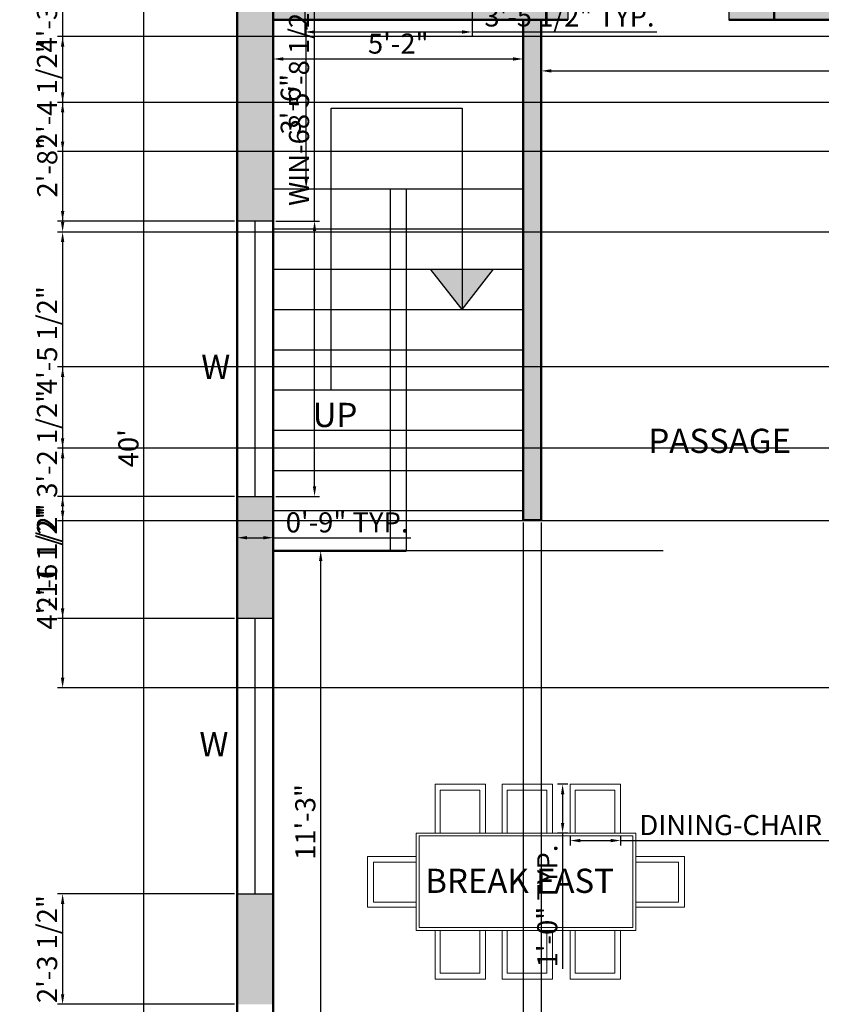
# Model space of a CAD drawing. Units: inches. Extents: x 2064 to 2999, y 1440 to 2089.
# Tile 2 of 7: x 2064 to 2263, y 1590 to 1835. Entities that reach past the tile are written whole.
import ezdxf

# ---------------------------------------------------------------- set-up
doc = ezdxf.new("R2010")
doc.units = ezdxf.units.IN
for name, color, linetype, lineweight in [('A-ANNO-DIMS', 2, 'Continuous', 18), ('A-ANNO-TEXT', 3, 'Continuous', 18), ('A-AREA-IDEN', 7, 'Continuous', 18), ('A-DOOR', 4, 'Continuous', 25), ('A-FLOR-STRS', 2, 'Continuous', 25), ('A-FURN', 8, 'Continuous', 18), ('A-GLAZ', 3, 'Continuous', 25), ('A-WALL', 7, 'Continuous', 50), ('A-WALL-PATT', 8, 'Continuous', 13)]:
    doc.layers.add(name, color=color, linetype=linetype, lineweight=lineweight)
doc.styles.get("Standard").update_dxf_attribs({"font": 'arial.ttf'})
doc.dimstyles.new('ISO-25', dxfattribs={"dimtxt": 5, "dimasz": 2.5, "dimexe": 1.25, "dimexo": 0.625, "dimtad": 1, "dimdec": 0, "dimlunit": 4, "dimtxsty": 'Standard', "dimcen": 2.5, "dimadec": 0, "dimazin": 0, "dimtfac": 1, "dimtdec": 0, "dimtmove": 0, "dimatfit": 3, "dimfxl": 1, "dimarcsym": 0})

# ---------------------------------------------------------------- blocks, each defined once
blk = doc.blocks.new('*U2')
for p, q in [((0, 0), (0, -6)), ((40, 0), (40, -6))]:
    blk.add_line(p, q)
blk.add_lwpolyline([(0, 0), (0, 40), (1.75, 40), (1.75, 0)], close=True)
blk.add_arc((0, 0), 40, 0, 90)
blk = doc.blocks.new('*D16')
at = {"layer": 'A-ANNO-DIMS', "color": 0, "lineweight": -2, "transparency": 16777216}
for p, q in [((2193.43, 1833.95), (2193.43, 1820.6)), ((2368.32, 1833.95), (2368.32, 1820.6)), ((2195.93, 1821.85), (2365.82, 1821.85))]:
    blk.add_line(p, q, dxfattribs=at)
at = {"layer": 'A-ANNO-DIMS', "color": 0, "transparency": 16777216}
for points in [[(2195.93, 1822.26), (2195.93, 1821.43), (2193.43, 1821.85)], [(2365.82, 1822.26), (2365.82, 1821.43), (2368.32, 1821.85)]]:
    blk.add_solid(points, dxfattribs=at)
at = {"layer": 'Defpoints', "color": 0, "transparency": 16777216}
for p in [(2193.43, 1834.57), (2368.32, 1834.57), (2368.32, 1821.85)]:
    blk.add_point(p, dxfattribs=at)
at = {"layer": 'A-ANNO-DIMS', "color": 0, "transparency": 16777216, "insert": (2280.88, 1824.98), "char_height": 5, "attachment_point": 5}
blk.add_mtext('14\'-7"', dxfattribs=at)
blk = doc.blocks.new('*D18')
at = {"layer": 'A-ANNO-DIMS', "color": 0, "lineweight": -2, "transparency": 16777216}
for p, q in [((2117.19, 1968.07), (2093.39, 1968.07)), ((2094.64, 1490.57), (2094.64, 1965.57)), ((2117.19, 1488.07), (2093.39, 1488.07))]:
    blk.add_line(p, q, dxfattribs=at)
at = {"layer": 'A-ANNO-DIMS', "color": 0, "transparency": 16777216}
for points in [[(2094.23, 1965.57), (2095.06, 1965.57), (2094.64, 1968.07)], [(2094.23, 1490.57), (2095.06, 1490.57), (2094.64, 1488.07)]]:
    blk.add_solid(points, dxfattribs=at)
at = {"layer": 'Defpoints', "color": 0, "transparency": 16777216}
for p in [(2094.64, 1968.07), (2117.82, 1968.07), (2117.82, 1488.07)]:
    blk.add_point(p, dxfattribs=at)
at = {"layer": 'A-ANNO-DIMS', "color": 0, "transparency": 16777216, "insert": (2091.47, 1728.07), "char_height": 5, "attachment_point": 5, "rotation": 90}
blk.add_mtext("40'", dxfattribs=at)
blk = doc.blocks.new('*D36')
at = {"layer": 'A-ANNO-DIMS', "color": 0, "lineweight": -2, "transparency": 16777216}
for p, q in [((2126.82, 1833.95), (2126.82, 1823.56)), ((2188.93, 1833.95), (2188.93, 1823.56)), ((2129.32, 1824.81), (2186.43, 1824.81))]:
    blk.add_line(p, q, dxfattribs=at)
at = {"layer": 'A-ANNO-DIMS', "color": 0, "transparency": 16777216}
for points in [[(2129.32, 1825.23), (2129.32, 1824.39), (2126.82, 1824.81)], [(2186.43, 1825.23), (2186.43, 1824.39), (2188.93, 1824.81)]]:
    blk.add_solid(points, dxfattribs=at)
at = {"layer": 'Defpoints', "color": 0, "transparency": 16777216}
for p in [(2126.82, 1834.57), (2188.93, 1834.57), (2188.93, 1824.81)]:
    blk.add_point(p, dxfattribs=at)
at = {"layer": 'A-ANNO-DIMS', "color": 0, "transparency": 16777216, "insert": (2157.88, 1827.99), "char_height": 5, "attachment_point": 5}
blk.add_mtext('5\'-2"', dxfattribs=at)
blk = doc.blocks.new('*D37')
at = {"layer": 'A-ANNO-DIMS', "color": 0, "lineweight": -2, "transparency": 16777216}
for p, q in [((2127.44, 1834.57), (2136.25, 1834.57)), ((2135, 1795.07), (2135, 1832.07)), ((2127.44, 1792.57), (2136.25, 1792.57))]:
    blk.add_line(p, q, dxfattribs=at)
at = {"layer": 'A-ANNO-DIMS', "color": 0, "transparency": 16777216}
for points in [[(2134.58, 1832.07), (2135.42, 1832.07), (2135, 1834.57)], [(2134.58, 1795.07), (2135.42, 1795.07), (2135, 1792.57)]]:
    blk.add_solid(points, dxfattribs=at)
at = {"layer": 'Defpoints', "color": 0, "transparency": 16777216}
for p in [(2126.82, 1834.57), (2135, 1834.57), (2126.82, 1792.57)]:
    blk.add_point(p, dxfattribs=at)
at = {"layer": 'A-ANNO-DIMS', "color": 0, "transparency": 16777216, "insert": (2131.82, 1813.57), "char_height": 5, "attachment_point": 5, "rotation": 90}
blk.add_mtext('3\'-6"', dxfattribs=at)
blk = doc.blocks.new('*D39')
at = {"layer": 'A-ANNO-DIMS', "color": 0, "lineweight": -2, "transparency": 16777216}
for p, q in [((2223.69, 1702.57), (2137.36, 1702.57)), ((2138.61, 1570.34), (2138.61, 1700.07)), ((2223.69, 1567.84), (2137.36, 1567.84))]:
    blk.add_line(p, q, dxfattribs=at)
at = {"layer": 'A-ANNO-DIMS', "color": 0, "transparency": 16777216}
for points in [[(2138.19, 1700.07), (2139.03, 1700.07), (2138.61, 1702.57)], [(2138.19, 1570.34), (2139.03, 1570.34), (2138.61, 1567.84)]]:
    blk.add_solid(points, dxfattribs=at)
at = {"layer": 'Defpoints', "color": 0, "transparency": 16777216}
for p in [(2138.61, 1702.57), (2224.32, 1702.57), (2224.32, 1567.84)]:
    blk.add_point(p, dxfattribs=at)
at = {"layer": 'A-ANNO-DIMS', "color": 0, "transparency": 16777216, "insert": (2135.43, 1635.2), "char_height": 5, "attachment_point": 5, "rotation": 90}
blk.add_mtext('11\'-3"', dxfattribs=at)
blk = doc.blocks.new('DINING-CHAIR')
for p, q in [((0, 0), (0, 12.53)), ((0, 12.53), (12.13, 12.53)), ((12.13, 0), (0, 0))]:
    blk.add_line(p, q)
blk.add_lwpolyline([(12.13, 11.12), (1.51, 11.12), (1.51, 1.24), (12.13, 1.24)], close=True)
blk = doc.blocks.new('WIN-68')
blk.add_line((4.5, 0), (4.5, 68.43))
blk.add_lwpolyline([(0, 0), (9, 0), (9, 68.43), (0, 68.43)], close=True)
blk = doc.blocks.new('*D50')
at = {"layer": 'A-ANNO-DIMS', "color": 0, "lineweight": -2, "transparency": 16777216}
for p, q in [((2134.69, 1838.45), (2134.69, 1830.27)), ((2176.26, 1838.45), (2176.26, 1830.27)), ((2137.19, 1831.52), (2173.76, 1831.52)), ((2176.26, 1831.52), (2222.13, 1831.52))]:
    blk.add_line(p, q, dxfattribs=at)
at = {"layer": 'A-ANNO-DIMS', "color": 0, "transparency": 16777216}
for points in [[(2137.19, 1831.93), (2137.19, 1831.1), (2134.69, 1831.52)], [(2173.76, 1831.93), (2173.76, 1831.1), (2176.26, 1831.52)]]:
    blk.add_solid(points, dxfattribs=at)
at = {"layer": 'Defpoints', "color": 0, "transparency": 16777216}
for p in [(2134.69, 1839.07), (2176.26, 1839.07), (2176.26, 1831.52)]:
    blk.add_point(p, dxfattribs=at)
at = {"layer": 'A-ANNO-DIMS', "color": 0, "transparency": 16777216, "insert": (2200.44, 1834.73), "char_height": 5, "attachment_point": 5}
blk.add_mtext('3\'-5 1/2" TYP.', dxfattribs=at)
blk = doc.blocks.new('*D57')
at = {"layer": 'A-ANNO-DIMS', "color": 0, "lineweight": -2, "transparency": 16777216}
for p, q in [((2200.61, 1631.83), (2200.61, 1629.33)), ((2203.11, 1630.58), (2210.65, 1630.58)), ((2213.15, 1631.83), (2213.15, 1629.33)), ((2213.15, 1630.58), (2309.22, 1630.58))]:
    blk.add_line(p, q, dxfattribs=at)
at = {"layer": 'A-ANNO-DIMS', "color": 0, "transparency": 16777216}
for points in [[(2203.11, 1631), (2203.11, 1630.16), (2200.61, 1630.58)], [(2210.65, 1631), (2210.65, 1630.16), (2213.15, 1630.58)]]:
    blk.add_solid(points, dxfattribs=at)
at = {"layer": 'Defpoints', "color": 0, "transparency": 16777216}
for p in [(2200.61, 1632.46), (2213.15, 1632.46), (2213.15, 1630.58)]:
    blk.add_point(p, dxfattribs=at)
at = {"layer": 'A-ANNO-DIMS', "color": 0, "transparency": 16777216, "insert": (2262.43, 1633.79), "char_height": 5, "attachment_point": 5}
blk.add_mtext('DINING-CHAIR 1\'-0 1/2" TYP.', dxfattribs=at)
blk = doc.blocks.new('*D58')
at = {"layer": 'A-ANNO-DIMS', "color": 0, "lineweight": -2, "transparency": 16777216}
for p, q in [((2199.99, 1644.59), (2197.48, 1644.59)), ((2198.73, 1642.09), (2198.73, 1634.96)), ((2199.99, 1632.46), (2197.48, 1632.46)), ((2198.73, 1632.46), (2198.73, 1598.7))]:
    blk.add_line(p, q, dxfattribs=at)
at = {"layer": 'A-ANNO-DIMS', "color": 0, "transparency": 16777216}
for points in [[(2198.32, 1642.09), (2199.15, 1642.09), (2198.73, 1644.59)], [(2198.32, 1634.96), (2199.15, 1634.96), (2198.73, 1632.46)]]:
    blk.add_solid(points, dxfattribs=at)
at = {"layer": 'Defpoints', "color": 0, "transparency": 16777216}
for p in [(2200.61, 1644.59), (2198.73, 1632.46), (2200.61, 1632.46)]:
    blk.add_point(p, dxfattribs=at)
at = {"layer": 'A-ANNO-DIMS', "color": 0, "transparency": 16777216, "insert": (2195.56, 1614.33), "char_height": 5, "attachment_point": 5, "rotation": 90}
blk.add_mtext('1\'-0" TYP.', dxfattribs=at)
blk = doc.blocks.new('*D59')
at = {"layer": 'A-ANNO-DIMS', "color": 0, "lineweight": -2, "transparency": 16777216}
for p, q in [((2137.08, 1784.53), (2137.08, 1856.23)), ((2127.44, 1784.53), (2138.33, 1784.53)), ((2137.08, 1718.6), (2137.08, 1782.03)), ((2127.44, 1716.1), (2138.33, 1716.1))]:
    blk.add_line(p, q, dxfattribs=at)
at = {"layer": 'A-ANNO-DIMS', "color": 0, "transparency": 16777216}
for points in [[(2136.67, 1782.03), (2137.5, 1782.03), (2137.08, 1784.53)], [(2136.67, 1718.6), (2137.5, 1718.6), (2137.08, 1716.1)]]:
    blk.add_solid(points, dxfattribs=at)
at = {"layer": 'Defpoints', "color": 0, "transparency": 16777216}
for p in [(2126.82, 1784.53), (2137.08, 1784.53), (2126.82, 1716.1)]:
    blk.add_point(p, dxfattribs=at)
at = {"layer": 'A-ANNO-DIMS', "color": 0, "transparency": 16777216, "insert": (2133.87, 1821.63), "char_height": 5, "attachment_point": 5, "rotation": 90}
blk.add_mtext('WIN-68 5\'-8 1/2" TYP.', dxfattribs=at)
blk = doc.blocks.new('*D60')
at = {"layer": 'A-ANNO-DIMS', "color": 0, "lineweight": -2, "transparency": 16777216}
for p, q in [((2117.82, 1715.48), (2117.82, 1704.59)), ((2126.82, 1715.48), (2126.82, 1704.59)), ((2120.32, 1705.84), (2124.32, 1705.84)), ((2126.82, 1705.84), (2161.05, 1705.84))]:
    blk.add_line(p, q, dxfattribs=at)
at = {"layer": 'A-ANNO-DIMS', "color": 0, "transparency": 16777216}
for points in [[(2120.32, 1706.25), (2120.32, 1705.42), (2117.82, 1705.84)], [(2124.32, 1706.25), (2124.32, 1705.42), (2126.82, 1705.84)]]:
    blk.add_solid(points, dxfattribs=at)
at = {"layer": 'Defpoints', "color": 0, "transparency": 16777216}
for p in [(2117.82, 1716.1), (2126.82, 1716.1), (2126.82, 1705.84)]:
    blk.add_point(p, dxfattribs=at)
at = {"layer": 'A-ANNO-DIMS', "color": 0, "transparency": 16777216, "insert": (2145.18, 1709.01), "char_height": 5, "attachment_point": 5}
blk.add_mtext('0\'-9" TYP.', dxfattribs=at)
blk = doc.blocks.new('*D70')
at = {"layer": 'A-ANNO-DIMS', "color": 0, "lineweight": -2, "transparency": 16777216}
for p, q in [((2477.19, 1865.66), (2073.22, 1865.66)), ((2074.47, 1863.16), (2074.47, 1816.51)), ((2477.19, 1814.01), (2073.22, 1814.01))]:
    blk.add_line(p, q, dxfattribs=at)
at = {"layer": 'A-ANNO-DIMS', "color": 0, "transparency": 16777216}
for points in [[(2074.05, 1863.16), (2074.89, 1863.16), (2074.47, 1865.66)], [(2074.05, 1816.51), (2074.89, 1816.51), (2074.47, 1814.01)]]:
    blk.add_solid(points, dxfattribs=at)
at = {"layer": 'Defpoints', "color": 0, "transparency": 16777216}
for p in [(2477.82, 1865.66), (2074.47, 1814.01), (2477.82, 1814.01)]:
    blk.add_point(p, dxfattribs=at)
at = {"layer": 'A-ANNO-DIMS', "color": 0, "transparency": 16777216, "insert": (2071.26, 1839.83), "char_height": 5, "attachment_point": 5, "rotation": 90}
blk.add_mtext('4\'-3 1/2"', dxfattribs=at)
blk = doc.blocks.new('*D71')
at = {"layer": 'A-ANNO-DIMS', "color": 0, "lineweight": -2, "transparency": 16777216}
for p, q in [((2477.19, 1814.01), (2073.22, 1814.01)), ((2074.47, 1811.51), (2074.47, 1784.3)), ((2477.19, 1781.8), (2073.22, 1781.8))]:
    blk.add_line(p, q, dxfattribs=at)
at = {"layer": 'A-ANNO-DIMS', "color": 0, "transparency": 16777216}
for points in [[(2074.05, 1811.51), (2074.89, 1811.51), (2074.47, 1814.01)], [(2074.05, 1784.3), (2074.89, 1784.3), (2074.47, 1781.8)]]:
    blk.add_solid(points, dxfattribs=at)
at = {"layer": 'Defpoints', "color": 0, "transparency": 16777216}
for p in [(2477.82, 1814.01), (2074.47, 1781.8), (2477.82, 1781.8)]:
    blk.add_point(p, dxfattribs=at)
at = {"layer": 'A-ANNO-DIMS', "color": 0, "transparency": 16777216, "insert": (2071.29, 1797.91), "char_height": 5, "attachment_point": 5, "rotation": 90}
blk.add_mtext('2\'-8"', dxfattribs=at)
blk = doc.blocks.new('*D72')
at = {"layer": 'A-ANNO-DIMS', "color": 0, "lineweight": -2, "transparency": 16777216}
for p, q in [((2477.19, 1781.8), (2073.22, 1781.8)), ((2074.47, 1779.3), (2074.47, 1730.57)), ((2477.19, 1728.07), (2073.22, 1728.07))]:
    blk.add_line(p, q, dxfattribs=at)
at = {"layer": 'A-ANNO-DIMS', "color": 0, "transparency": 16777216}
for points in [[(2074.05, 1779.3), (2074.89, 1779.3), (2074.47, 1781.8)], [(2074.05, 1730.57), (2074.89, 1730.57), (2074.47, 1728.07)]]:
    blk.add_solid(points, dxfattribs=at)
at = {"layer": 'Defpoints', "color": 0, "transparency": 16777216}
for p in [(2477.82, 1781.8), (2074.47, 1728.07), (2477.82, 1728.07)]:
    blk.add_point(p, dxfattribs=at)
at = {"layer": 'A-ANNO-DIMS', "color": 0, "transparency": 16777216, "insert": (2071.26, 1754.94), "char_height": 5, "attachment_point": 5, "rotation": 90}
blk.add_mtext('4\'-5 1/2"', dxfattribs=at)
blk = doc.blocks.new('*D73')
at = {"layer": 'A-ANNO-DIMS', "color": 0, "lineweight": -2, "transparency": 16777216}
for p, q in [((2477.19, 1728.07), (2073.22, 1728.07)), ((2074.47, 1725.57), (2074.47, 1671.03)), ((2477.19, 1668.53), (2073.22, 1668.53))]:
    blk.add_line(p, q, dxfattribs=at)
at = {"layer": 'A-ANNO-DIMS', "color": 0, "transparency": 16777216}
for points in [[(2074.05, 1725.57), (2074.89, 1725.57), (2074.47, 1728.07)], [(2074.05, 1671.03), (2074.89, 1671.03), (2074.47, 1668.53)]]:
    blk.add_solid(points, dxfattribs=at)
at = {"layer": 'Defpoints', "color": 0, "transparency": 16777216}
for p in [(2477.82, 1728.07), (2074.47, 1668.53), (2477.82, 1668.53)]:
    blk.add_point(p, dxfattribs=at)
at = {"layer": 'A-ANNO-DIMS', "color": 0, "transparency": 16777216, "insert": (2071.26, 1698.3), "char_height": 5, "attachment_point": 5, "rotation": 90}
blk.add_mtext('4\'-11 1/2"', dxfattribs=at)
blk = doc.blocks.new('*D74')
at = {"layer": 'A-ANNO-DIMS', "color": 0, "lineweight": -2, "transparency": 16777216}
for p, q in [((2117.19, 1968.07), (2073.22, 1968.07)), ((2074.47, 1965.57), (2074.47, 1787.03)), ((2117.19, 1784.53), (2073.22, 1784.53))]:
    blk.add_line(p, q, dxfattribs=at)
at = {"layer": 'A-ANNO-DIMS', "color": 0, "transparency": 16777216}
for points in [[(2074.05, 1965.57), (2074.89, 1965.57), (2074.47, 1968.07)], [(2074.05, 1787.03), (2074.89, 1787.03), (2074.47, 1784.53)]]:
    blk.add_solid(points, dxfattribs=at)
at = {"layer": 'Defpoints', "color": 0, "transparency": 16777216}
for p in [(2117.82, 1968.07), (2074.47, 1784.53), (2117.82, 1784.53)]:
    blk.add_point(p, dxfattribs=at)
at = {"layer": 'A-ANNO-DIMS', "color": 0, "transparency": 16777216, "insert": (2071.26, 1876.3), "char_height": 5, "attachment_point": 5, "rotation": 90}
blk.add_mtext('15\'-3 1/2"', dxfattribs=at)
blk = doc.blocks.new('*D75')
at = {"layer": 'A-ANNO-DIMS', "color": 0, "lineweight": -2, "transparency": 16777216}
for p, q in [((2117.19, 1716.1), (2073.22, 1716.1)), ((2074.47, 1713.6), (2074.47, 1688.26)), ((2117.19, 1685.76), (2073.22, 1685.76))]:
    blk.add_line(p, q, dxfattribs=at)
at = {"layer": 'A-ANNO-DIMS', "color": 0, "transparency": 16777216}
for points in [[(2074.05, 1713.6), (2074.89, 1713.6), (2074.47, 1716.1)], [(2074.05, 1688.26), (2074.89, 1688.26), (2074.47, 1685.76)]]:
    blk.add_solid(points, dxfattribs=at)
at = {"layer": 'Defpoints', "color": 0, "transparency": 16777216}
for p in [(2117.82, 1716.1), (2074.47, 1685.76), (2117.82, 1685.76)]:
    blk.add_point(p, dxfattribs=at)
at = {"layer": 'A-ANNO-DIMS', "color": 0, "transparency": 16777216, "insert": (2071.26, 1700.93), "char_height": 5, "attachment_point": 5, "rotation": 90}
blk.add_mtext('2\'-6 1/2"', dxfattribs=at)
blk = doc.blocks.new('*D76')
at = {"layer": 'A-ANNO-DIMS', "color": 0, "lineweight": -2, "transparency": 16777216}
for p, q in [((2117.19, 1617.33), (2073.22, 1617.33)), ((2074.47, 1614.83), (2074.47, 1592.39)), ((2117.19, 1589.89), (2073.22, 1589.89))]:
    blk.add_line(p, q, dxfattribs=at)
at = {"layer": 'A-ANNO-DIMS', "color": 0, "transparency": 16777216}
for points in [[(2074.05, 1614.83), (2074.89, 1614.83), (2074.47, 1617.33)], [(2074.05, 1592.39), (2074.89, 1592.39), (2074.47, 1589.89)]]:
    blk.add_solid(points, dxfattribs=at)
at = {"layer": 'Defpoints', "color": 0, "transparency": 16777216}
for p in [(2117.82, 1617.33), (2074.47, 1589.89), (2117.82, 1589.89)]:
    blk.add_point(p, dxfattribs=at)
at = {"layer": 'A-ANNO-DIMS', "color": 0, "transparency": 16777216, "insert": (2071.26, 1603.61), "char_height": 5, "attachment_point": 5, "rotation": 90}
blk.add_mtext('2\'-3 1/2"', dxfattribs=at)
blk = doc.blocks.new('*D96')
at = {"layer": 'A-ANNO-DIMS', "color": 0, "lineweight": -2, "transparency": 16777216}
for p, q in [((2188.93, 1709.59), (2188.93, 1443.47)), ((2193.43, 1709.59), (2193.43, 1443.47)), ((2186.43, 1444.72), (2183.93, 1444.72)), ((2188.93, 1444.72), (2193.43, 1444.72)), ((2195.93, 1444.72), (2224.63, 1444.72))]:
    blk.add_line(p, q, dxfattribs=at)
at = {"layer": 'A-ANNO-DIMS', "color": 0, "transparency": 16777216}
for points in [[(2186.43, 1445.14), (2186.43, 1444.3), (2188.93, 1444.72)], [(2195.93, 1445.14), (2195.93, 1444.3), (2193.43, 1444.72)]]:
    blk.add_solid(points, dxfattribs=at)
at = {"layer": 'Defpoints', "color": 0, "transparency": 16777216}
for p in [(2188.93, 1710.22), (2193.43, 1710.22), (2193.43, 1444.72)]:
    blk.add_point(p, dxfattribs=at)
at = {"layer": 'A-ANNO-DIMS', "color": 0, "transparency": 16777216, "insert": (2211.53, 1447.93), "char_height": 5, "attachment_point": 5}
blk.add_mtext('0\'-4 1/2"', dxfattribs=at)
blk = doc.blocks.new('*D113')
at = {"layer": 'A-ANNO-DIMS', "color": 0, "lineweight": -2, "transparency": 16777216}
for p, q in [((2372.19, 1830.37), (2073.22, 1830.37)), ((2074.47, 1827.87), (2074.47, 1804.28)), ((2372.19, 1801.78), (2073.22, 1801.78))]:
    blk.add_line(p, q, dxfattribs=at)
at = {"layer": 'A-ANNO-DIMS', "color": 0, "transparency": 16777216}
for points in [[(2074.05, 1827.87), (2074.89, 1827.87), (2074.47, 1830.37)], [(2074.05, 1804.28), (2074.89, 1804.28), (2074.47, 1801.78)]]:
    blk.add_solid(points, dxfattribs=at)
at = {"layer": 'Defpoints', "color": 0, "transparency": 16777216}
for p in [(2372.82, 1830.37), (2074.47, 1801.78), (2372.82, 1801.78)]:
    blk.add_point(p, dxfattribs=at)
at = {"layer": 'A-ANNO-DIMS', "color": 0, "transparency": 16777216, "insert": (2071.26, 1816.07), "char_height": 5, "attachment_point": 5, "rotation": 90}
blk.add_mtext('2\'-4 1/2"', dxfattribs=at)
blk = doc.blocks.new('*D114')
at = {"layer": 'A-ANNO-DIMS', "color": 0, "lineweight": -2, "transparency": 16777216}
for p, q in [((2349.69, 1748.3), (2073.22, 1748.3)), ((2074.47, 1745.8), (2074.47, 1712.55)), ((2348.19, 1710.05), (2073.22, 1710.05))]:
    blk.add_line(p, q, dxfattribs=at)
at = {"layer": 'A-ANNO-DIMS', "color": 0, "transparency": 16777216}
for points in [[(2074.05, 1745.8), (2074.89, 1745.8), (2074.47, 1748.3)], [(2074.05, 1712.55), (2074.89, 1712.55), (2074.47, 1710.05)]]:
    blk.add_solid(points, dxfattribs=at)
at = {"layer": 'Defpoints', "color": 0, "transparency": 16777216}
for p in [(2350.32, 1748.3), (2074.47, 1710.05), (2348.82, 1710.05)]:
    blk.add_point(p, dxfattribs=at)
at = {"layer": 'A-ANNO-DIMS', "color": 0, "transparency": 16777216, "insert": (2071.26, 1729.18), "char_height": 5, "attachment_point": 5, "rotation": 90}
blk.add_mtext('3\'-2 1/2"', dxfattribs=at)

msp = doc.modelspace()

# ---------------------------------------------------------------- hatches: boundary and pattern name
at = {"layer": 'A-FLOR-STRS'}
h = msp.add_hatch(color=256, dxfattribs=at)
h.dxf.hatch_style = 1
h.paths.add_polyline_path([(2173.73, 1772.57), (2165.88, 1772.57), (2173.73, 1762.57)])
h.paths.add_polyline_path([(2181.59, 1772.57), (2173.73, 1772.57), (2173.73, 1762.57)])
at = {"layer": 'A-WALL-PATT'}
h = msp.add_hatch(color=256, dxfattribs=at)
h.dxf.hatch_style = 1
h.paths.add_polyline_path([(2267.27, 1968.07), (2215.88, 1968.07), (2215.88, 1959.07), (2246.82, 1959.07), (2267.27, 1959.07)])
h.paths.add_polyline_path([(2477.82, 1968.07), (2300.73, 1968.07), (2300.73, 1959.07), (2317.32, 1959.07), (2468.82, 1959.07), (2468.82, 1925.2), (2477.82, 1925.2)])
h.paths.add_polyline_path([(2154.1, 1968.07), (2117.82, 1968.07), (2117.82, 1784.53), (2126.82, 1784.53), (2126.82, 1959.07), (2154.1, 1959.07)])
h.paths.add_polyline_path([(2126.82, 1716.1), (2117.82, 1716.1), (2117.82, 1685.76), (2126.82, 1685.76)])
h.paths.add_polyline_path([(2126.82, 1617.33), (2117.82, 1617.33), (2117.82, 1589.89), (2126.82, 1589.89)])
h.paths.add_polyline_path([(2273.05, 1497.07), (2228.82, 1497.07), (2126.82, 1497.07), (2126.82, 1521.07), (2126.82, 1521.46), (2117.82, 1521.46), (2117.82, 1488.07), (2273.05, 1488.07)])
h.paths.add_polyline_path([(2409.19, 1494.07, -0.01877), (2409.3, 1497.07), (2356.92, 1497.07), (2356.92, 1488.07), (2409.19, 1488.07)])
h.paths.add_polyline_path([(2468.82, 1638.07), (2348.82, 1638.07), (2348.82, 1668.53), (2348.82, 1710.05), (2344.32, 1710.05), (2344.32, 1633.57), (2468.82, 1633.57)])
h.paths.add_polyline_path([(2228.82, 1567.84), (2224.32, 1567.84), (2224.32, 1497.07), (2228.82, 1497.07)])
h.paths.add_polyline_path([(2477.82, 1781.8), (2468.82, 1781.8), (2468.82, 1762.57), (2468.82, 1728.07), (2477.82, 1728.07)])
h.paths.add_polyline_path([(2468.82, 1762.57), (2372.82, 1762.57), (2372.82, 1801.78), (2368.32, 1801.78), (2368.32, 1758.07), (2468.82, 1758.07)])
h.paths.add_polyline_path([(2477.82, 1865.66), (2468.82, 1865.66), (2468.82, 1814.01), (2477.82, 1814.01)])
h.paths.add_polyline_path([(2321.82, 1959.07), (2317.32, 1959.07), (2317.32, 1839.07), (2251.32, 1839.07), (2251.32, 1834.57), (2321.82, 1834.57)])
h.paths.add_polyline_path([(2200.07, 1839.07), (2126.82, 1839.07), (2126.82, 1834.57), (2200.07, 1834.57)])
h.paths.add_polyline_path([(2193.43, 1834.57), (2188.93, 1834.57), (2188.93, 1710.22), (2193.43, 1710.22)])
h.paths.add_polyline_path([(2251.32, 1959.07), (2246.82, 1959.07), (2246.82, 1950.75), (2251.21, 1950.75), (2251.32, 1950.75)])
h.paths.add_polyline_path([(2251.32, 1921.46), (2246.82, 1921.46), (2246.82, 1839.07), (2240.07, 1839.07), (2240.07, 1834.57), (2251.32, 1834.57), (2251.32, 1839.07)])
h.paths.add_polyline_path([(2468.82, 1839.07), (2363.36, 1839.07), (2363.36, 1834.57), (2468.82, 1834.57)])
h.paths.add_polyline_path([(2323.36, 1839.07), (2321.82, 1839.07), (2321.82, 1834.57), (2323.36, 1834.57)])
h = msp.add_hatch(color=256, dxfattribs=at)
h.dxf.hatch_style = 1
h.paths.add_polyline_path([(2449.19, 1497.07), (2449.19, 1494.07), (2449.19, 1488.07), (2468.82, 1488.07), (2468.82, 1497.07)])
h.paths.add_polyline_path([(2468.82, 1488.07), (2477.82, 1488.07), (2477.82, 1668.53), (2468.82, 1668.53)])
h.paths.add_polyline_path([(2454.62, 1692.05), (2454.62, 1703.66), (2444.32, 1703.66), (2444.32, 1692.05)], flags=9)
h.paths.add_polyline_path([(2167.39, 1527.81), (2183.8, 1527.81), (2183.8, 1538.12), (2167.39, 1538.12)], flags=9)
h.paths.add_polyline_path([(2343.08, 1527.75), (2354.68, 1527.75), (2354.68, 1538.06), (2343.08, 1538.06)], flags=9)
h.paths.add_polyline_path([(2462.54, 1554.96), (2462.54, 1575.25), (2452.24, 1575.25), (2452.24, 1554.96)], flags=9)
h.paths.add_polyline_path([(2140.63, 1624.84), (2140.63, 1645.13), (2130.32, 1645.13), (2130.32, 1624.84)], flags=9)
h.paths.add_polyline_path([(2137.9, 1938.01), (2190.4, 1938.01), (2190.4, 1950.4), (2137.9, 1950.4)], flags=9)
h.paths.add_polyline_path([(2337.44, 1898.9), (2337.44, 1951.39), (2325.04, 1951.39), (2325.04, 1898.9)], flags=9)
h.paths.add_polyline_path([(2380.15, 1768.58), (2405.57, 1768.58), (2405.57, 1780.97), (2380.15, 1780.97)], flags=9)
h.paths.add_polyline_path([(2370.32, 1679.42), (2432.16, 1679.42), (2432.16, 1691.82), (2370.32, 1691.82)], flags=9)
h.paths.add_polyline_path([(2322.2, 1541.98), (2382.63, 1541.98), (2382.63, 1554.37), (2322.2, 1554.37)], flags=9)
h.paths.add_polyline_path([(2153.83, 1534.75), (2193.72, 1534.75), (2193.72, 1547.14), (2153.83, 1547.14)], flags=9)
h.paths.add_polyline_path([(2162.47, 1614.19), (2217.78, 1614.19), (2217.78, 1626.58), (2162.47, 1626.58)], flags=9)
h.paths.add_polyline_path([(2217.9, 1723.52), (2261.07, 1723.52), (2261.07, 1735.92), (2217.9, 1735.92)], flags=9)
h.paths.add_polyline_path([(2270.61, 1869.16), (2296.03, 1869.16), (2296.03, 1881.55), (2270.61, 1881.55)], flags=9)
h.paths.add_polyline_path([(2353.7, 1922), (2422.07, 1922), (2422.07, 1934.4), (2353.7, 1934.4)], flags=9)
h.paths.add_polyline_path([(2133.7, 1917.44), (2217.48, 1917.44), (2217.48, 1929.83), (2133.7, 1929.83)], flags=9)

# ---------------------------------------------------------------- linework, layer by layer
at = {"layer": 'A-FLOR-STRS'}
for p, q in [((2141.24, 1742.57), (2141.24, 1812.55)), ((2141.24, 1812.55), (2173.73, 1812.55)), ((2173.73, 1812.55), (2173.73, 1762.57)), ((2126.82, 1792.57), (2188.93, 1792.57)), ((2155.88, 1792.57), (2155.88, 1714.15)), ((2159.88, 1792.57), (2159.88, 1714.15)), ((2126.82, 1782.57), (2188.93, 1782.57)), ((2126.82, 1772.57), (2188.93, 1772.57)), ((2173.73, 1762.57), (2165.88, 1772.57)), ((2173.73, 1762.57), (2181.59, 1772.57)), ((2126.82, 1762.57), (2188.93, 1762.57)), ((2126.82, 1752.57), (2188.93, 1752.57)), ((2126.82, 1742.57), (2188.93, 1742.57)), ((2126.82, 1732.57), (2188.93, 1732.57)), ((2126.82, 1722.57), (2188.93, 1722.57)), ((2155.88, 1714.15), (2155.88, 1702.57)), ((2159.88, 1714.15), (2159.88, 1702.57)), ((2126.82, 1712.57), (2188.93, 1712.57))]:
    msp.add_line(p, q, dxfattribs=at)
at = {"layer": 'A-FURN'}
for points in [[(2162.37, 1608.23), (2216.93, 1608.23), (2216.93, 1632.46), (2162.37, 1632.46)], [(2163.08, 1608.94), (2216.22, 1608.94), (2216.22, 1631.75), (2163.08, 1631.75)]]:
    msp.add_lwpolyline(points, close=True, dxfattribs=at)
at = {"layer": 'A-WALL'}
for p, q in [((2117.82, 1488.07), (2117.82, 1968.07)), ((2251.32, 1921.46), (2251.32, 1834.57)), ((2200.07, 1834.57), (2126.82, 1834.57)), ((2126.82, 1834.57), (2126.82, 1792.57)), ((2188.93, 1710.22), (2188.93, 1834.57)), ((2193.43, 1834.57), (2193.43, 1710.22)), ((2251.32, 1834.57), (2240.07, 1834.57)), ((2321.82, 1834.57), (2251.32, 1834.57)), ((2193.43, 1710.22), (2188.93, 1710.22)), ((2126.82, 1702.57), (2159.88, 1702.57))]:
    msp.add_line(p, q, dxfattribs=at)
for points in [[(2449.19, 1488.07), (2477.82, 1488.07), (2477.82, 1968.07), (2117.82, 1968.07), (2117.82, 1488.07), (2409.19, 1488.07)], [(2447.44, 1497.07), (2468.82, 1497.07), (2468.82, 1959.07), (2126.82, 1959.07), (2126.82, 1497.07), (2409.3, 1497.07)]]:
    msp.add_lwpolyline(points, dxfattribs=at)

# ---------------------------------------------------------------- block references
at = {"layer": 'A-DOOR', "xscale": -1}
msp.add_blockref('*U2', (2240.07, 1840.57), dxfattribs=at)
at = {"layer": 'A-FURN'}
for p, rotation in [((2167.07, 1644.59), 270.000000000004), ((2183.72, 1644.59), 270.000000000004), ((2200.61, 1644.59), 270.0000000000001)]:
    msp.add_blockref('DINING-CHAIR', p, dxfattribs=dict(at, rotation=rotation))
msp.add_blockref('DINING-CHAIR', (2150.24, 1614.06), dxfattribs=at)
at = {"layer": 'A-FURN', "extrusion": (0, 0, -1), "zscale": -1}
msp.add_blockref('DINING-CHAIR', (-2229.06, 1614.06), dxfattribs=at)
for p, rotation in [((-2167.07, 1596.1), 90.00000000000193), ((-2183.72, 1596.1), 90.00000000000193), ((-2200.61, 1596.1), 89.99999999999805)]:
    msp.add_blockref('DINING-CHAIR', p, dxfattribs=dict(at, rotation=rotation))
at = {"layer": 'A-GLAZ'}
for p in [(2117.82, 1716.1), (2117.82, 1617.33)]:
    msp.add_blockref('WIN-68', p, dxfattribs=at)

# ---------------------------------------------------------------- texts
at = {"layer": 'A-ANNO-TEXT', "char_height": 6.02, "attachment_point": 1}
for insert in [(2108.92, 1751.29), (2108.46, 1657.56)]:
    msp.add_mtext_dynamic_manual_height_columns('W', width=152.6727, gutter_width=30.08, heights=[0], dxfattribs=dict(at, insert=insert))
at = {"layer": 'A-AREA-IDEN', "char_height": 6.015, "attachment_point": 1}
for s, insert in [('UP', (2136.61, 1739.36)), ('PASSAGE', (2220.05, 1732.92)), ('BREAK FAST', (2164.59, 1623.59))]:
    msp.add_mtext_dynamic_manual_height_columns(s, width=152.6727, gutter_width=30.08, heights=[0], dxfattribs=dict(at, insert=insert))

# ---------------------------------------------------------------- dimensions: what is measured, and where the dimension line sits
at = {"layer": 'A-ANNO-DIMS'}
for base, p1, p2, override, picture, middle in [((2074.47, 1784.53), (2117.82, 1968.07), (2117.82, 1784.53), {"dimdec": 1, "dimlfac": 1, "dimrnd": 0, "dimzin": 1, "dimdsep": 46, "dimlunit": 4, "dimfrac": 2}, '*D74', (2071.26, 1876.3)), ((2094.64, 1968.07), (2117.82, 1488.07), (2117.82, 1968.07), {"dimclrd": 0, "dimclre": 0, "dimclrt": 0}, '*D18', (2091.47, 1728.07)), ((2074.4687, 1814.0143), (2477.8187, 1865.6554), (2477.8187, 1814.0143), {"dimdec": 1, "dimlfac": 1, "dimrnd": 0, "dimzin": 1, "dimdsep": 46, "dimlunit": 4, "dimfrac": 2}, '*D70', (2071.2567, 1839.8348)), ((2135, 1834.57), (2126.82, 1792.57), (2126.82, 1834.57), {"dimclrd": 0, "dimclre": 0, "dimclrt": 0}, '*D37', (2131.82, 1813.57)), ((2074.47, 1801.78), (2372.82, 1830.37), (2372.82, 1801.78), {"dimdec": 1, "dimlfac": 1, "dimrnd": 0, "dimzin": 1, "dimdsep": 46, "dimlunit": 4, "dimfrac": 2}, '*D113', (2071.26, 1816.07)), ((2074.47, 1781.8), (2477.82, 1814.01), (2477.82, 1781.8), {"dimdec": 1, "dimlfac": 1, "dimrnd": 0, "dimzin": 1, "dimdsep": 46, "dimlunit": 4, "dimfrac": 2}, '*D71', (2071.29, 1797.91)), ((2074.47, 1728.07), (2477.82, 1781.8), (2477.82, 1728.07), {"dimdec": 1, "dimlfac": 1, "dimrnd": 0, "dimzin": 1, "dimdsep": 46, "dimlunit": 4, "dimfrac": 2}, '*D72', (2071.26, 1754.94)), ((2074.468681, 1710.052363), (2350.318681, 1748.302363), (2348.818681, 1710.052363), {"dimdec": 1, "dimlfac": 1, "dimrnd": 0, "dimzin": 1, "dimdsep": 46, "dimlunit": 4, "dimfrac": 2}, '*D114', (2071.25670965, 1729.177363)), ((2074.47, 1668.53), (2477.82, 1728.07), (2477.82, 1668.53), {"dimdec": 1, "dimlfac": 1, "dimrnd": 0, "dimzin": 1, "dimdsep": 46, "dimlunit": 4, "dimfrac": 2}, '*D73', (2071.26, 1698.3)), ((2074.47, 1685.76), (2117.82, 1716.1), (2117.82, 1685.76), {"dimdec": 1, "dimlfac": 1, "dimrnd": 0, "dimzin": 1, "dimdsep": 46, "dimlunit": 4, "dimfrac": 2}, '*D75', (2071.26, 1700.93)), ((2138.61, 1702.57), (2224.32, 1567.84), (2224.32, 1702.57), {"dimclrd": 0, "dimclre": 0, "dimclrt": 0}, '*D39', (2135.43, 1635.2)), ((2074.47, 1589.89), (2117.82, 1617.33), (2117.82, 1589.89), {"dimdec": 1, "dimlfac": 1, "dimrnd": 0, "dimzin": 1, "dimdsep": 46, "dimlunit": 4, "dimfrac": 2}, '*D76', (2071.26, 1603.61))]:
    dim = msp.add_linear_dim(base=base, p1=p1, p2=p2, angle=90, dimstyle='ISO-25', override=override, dxfattribs=at)
    dim.commit()
    dim.dimension.update_dxf_attribs({"geometry": picture, "text_midpoint": middle})
for base, p1, p2, angle, text, picture, middle in [((2137.08, 1784.53), (2126.82, 1716.1), (2126.82, 1784.53), 90, 'WIN-68 <> TYP.', '*D59', (2133.87, 1821.63)), ((2198.73, 1632.46), (2200.61, 1644.59), (2200.61, 1632.46), 270, '<> TYP.', '*D58', (2195.56, 1614.33))]:
    dim = msp.add_linear_dim(base=base, p1=p1, p2=p2, angle=angle, text=text, dimstyle='ISO-25', override={"dimdec": 1, "dimrnd": 0, "dimzin": 1, "dimlunit": 4, "dimfrac": 2}, dxfattribs=at)
    dim.commit()
    dim.dimension.update_dxf_attribs({"geometry": picture, "text_midpoint": middle})
for base, p1, p2, text, picture, middle in [((2176.26, 1831.52), (2134.69, 1839.07), (2176.26, 1839.07), '<> TYP.', '*D50', (2200.44, 1834.73)), ((2126.82, 1705.84), (2117.82, 1716.1), (2126.82, 1716.1), '<> TYP.', '*D60', (2145.18, 1709.01)), ((2213.15, 1630.58), (2200.61, 1632.46), (2213.15, 1632.46), 'DINING-CHAIR <> TYP.', '*D57', (2262.43, 1633.79))]:
    dim = msp.add_linear_dim(base=base, p1=p1, p2=p2, text=text, dimstyle='ISO-25', override={"dimdec": 1, "dimrnd": 0, "dimzin": 1, "dimlunit": 4, "dimfrac": 2}, dxfattribs=at)
    dim.commit()
    dim.dimension.update_dxf_attribs({"geometry": picture, "text_midpoint": middle})
for base, p1, p2, override, picture, middle in [((2188.93, 1824.81), (2126.82, 1834.57), (2188.93, 1834.57), {"dimclrd": 0, "dimclre": 0, "dimclrt": 0}, '*D36', (2157.88, 1827.99)), ((2368.32, 1821.85), (2193.43, 1834.57), (2368.32, 1834.57), {"dimclrd": 0, "dimclre": 0, "dimclrt": 0}, '*D16', (2280.88, 1824.98)), ((2193.43, 1444.72), (2188.93, 1710.22), (2193.43, 1710.22), {"dimdec": 1, "dimlfac": 1, "dimrnd": 0, "dimzin": 1, "dimdsep": 46, "dimlunit": 4, "dimfrac": 2}, '*D96', (2211.53, 1447.93))]:
    dim = msp.add_linear_dim(base=base, p1=p1, p2=p2, dimstyle='ISO-25', override=override, dxfattribs=at)
    dim.commit()
    dim.dimension.update_dxf_attribs({"geometry": picture, "text_midpoint": middle})

doc.saveas('drawing.dxf')
